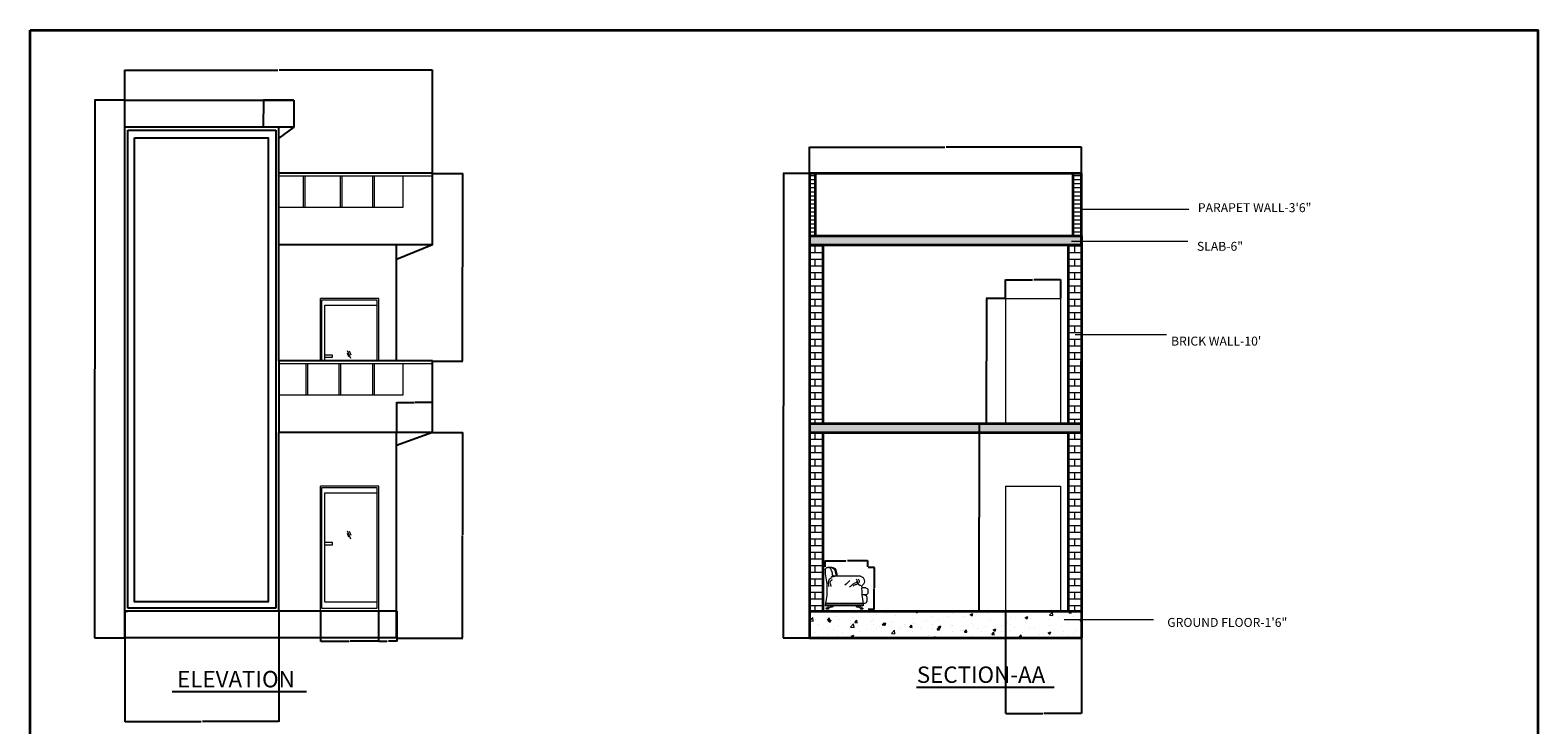
# Model space of a CAD drawing. Units: inches. Extents: x 2169 to 3181, y 1824 to 2912.
# Tile 5 of 5: x 2169 to 3181, y 2446 to 2912. Entities that reach past the tile are written whole.
import ezdxf

# ---------------------------------------------------------------- set-up
doc = ezdxf.new("R2010")
doc.units = ezdxf.units.IN
for name, color, linetype, lineweight in [('A-ANNO-DIMS', 2, 'Continuous', 18), ('A-ANNO-TEXT', 7, 'Continuous', 18), ('A-ANNO-TITL', 7, 'Continuous', 25), ('A-ANNO-TTLB', 7, 'Continuous', 35), ('A-DOOR-ELEV', 3, 'Continuous', 18), ('A-ELEV', 7, 'Continuous', 25), ('A-ELEV-RAIL', 7, 'Continuous', 18), ('A-FLOR-PATT', 252, 'Continuous', 13), ('A-FURN', 8, 'Continuous', 18), ('A-SECT', 7, 'Continuous', 35), ('A-SECT-PRJE', 7, 'Continuous', 18), ('A-WALL-PATT', 252, 'Continuous', 13)]:
    doc.layers.add(name, color=color, linetype=linetype, lineweight=lineweight)
doc.styles.get("Standard").update_dxf_attribs({"font": 'arial.ttf'})
doc.dimstyles.get("Standard").update_dxf_attribs({"dimtxt": 0.18, "dimasz": 0.18, "dimexe": 0.18, "dimexo": 0.0625, "dimgap": 0.09, "dimtad": 0, "dimtih": 1, "dimtoh": 1, "dimdec": 4, "dimzin": 0, "dimdsep": 46, "dimtxsty": 'Standard', "dimcen": 0.09, "dimadec": 0, "dimazin": 0, "dimtfac": 1, "dimtdec": 4, "dimtofl": 0, "dimtmove": 0, "dimatfit": 3, "dimfxl": 1, "dimtolj": 1, "dimtzin": 0, "dimarcsym": 0})

# ---------------------------------------------------------------- blocks, each defined once
blk = doc.blocks.new('A$C624B6646')
for p, q in [((153, 697), (704, 697)), ((161, 698), (700, 698)), ((700, 688), (780, 668)), ((738, 711), (780, 668)), ((769, 889), (830, 881)), ((830, 881), (850, 881)), ((900, 831), (900, 745)), ((0, 400), (0, 350)), ((50, 450), (132, 450)), ((23, 250), (23, 170)), ((50, 300), (125, 300)), ((73, 120), (100, 120)), ((100, 120), (100, 82)), ((100, 82), (900, 82)), ((100, 82), (100, 70)), ((100, 70), (900, 70)), ((104, 120), (900, 120)), ((113, 1), (156, 0)), ((157, 12), (156, 0)), ((166, 27), (157, 12)), ((260, 82), (239, 50)), ((729, 82), (750, 50)), ((823, 27), (832, 12)), ((832, 12), (834, 0)), ((834, 0), (876, 1)), ((900, 82), (900, 70))]:
    blk.add_line(p, q)
for centre, radius, start, end in [((183, 593), 109, 106.2053, 229.88), ((1468, 575), 827, 165.0137, 171.498), ((769, 789), 100, 90, 180), ((1490, 575), 827, 165.0137, 171.498), ((799, 781), 108, 99.7535, 175.837), ((704, 747), 50, 270, 355.0653), ((983, 723), 230, 152.1091, 175.0653), ((830, 831), 50, 90, 180), ((850, 831), 50, 0, 90), ((50, 400), 50, 90, 180), ((50, 350), 50, 180, 270), ((81, 471), 50, 1.791, 49.88), ((73, 250), 50, 90, 180), ((73, 170), 50, 180, 270), ((97, 118), 97.9, 273.831, 296.417), ((118, 16), 15.5, 163.7636, 251.7535), ((230, -4), 95.2, 115.8946, 159.312), ((224, -28), 79.9, 78.8551, 136.1209), ((765, -28), 79.9, 43.8791, 101.1449), ((760, -4), 95.2, 20.688, 64.1054), ((893, 118), 97.9, 243.583, 266.169), ((871, 16), 15.5, 288.2465, 16.2364)]:
    blk.add_arc(centre, radius, start, end)
for points, knots in [([(203, 637), (194, 624), (167, 587), (216, 515), (280, 515), (306, 492), (315, 484)], [0, 0, 0, 0, 46.783568, 128.12179, 194.346234, 229.237423, 229.237423, 229.237423, 229.237423]), ([(245, 644), (235, 621), (212, 571), (298, 543), (345, 504), (373, 475), (385, 463)], [0, 0, 0, 0, 64.284597, 139.770948, 209.553279, 258.887454, 258.887454, 258.887454, 258.887454]), ([(774, 650), (789, 644), (834, 629), (840, 550), (833, 502), (830, 482)], [0, 0, 0, 0, 46.821513, 133.069671, 196.206665, 196.206665, 196.206665, 196.206665]), ([(900, 745), (882, 634), (846, 413), (882, 192), (900, 82)], [0, 0, 0, 0, 336.072717, 666.841786, 666.841786, 666.841786, 666.841786]), ([(147, 498), (162, 501), (194, 507), (223, 553), (219, 586), (217, 602)], [0, 0, 0, 0, 44.149611, 94.447762, 143.253115, 143.253115, 143.253115, 143.253115]), ([(753, 622), (775, 607), (818, 579), (789, 521), (783, 491), (781, 482)], [0, 0, 0, 0, 69.067804, 133.352323, 162.101735, 162.101735, 162.101735, 162.101735])]:
    blk.add_open_spline(points, degree=3, knots=knots)
for points in [[(131, 473), (135, 356), (120, 238), (104, 120)], [(378, 609), (415, 575), (452, 540), (489, 505)]]:
    blk.add_open_spline(points, degree=3)
blk = doc.blocks.new('A$C4C705FAE')
blk.add_blockref('A$C624B6646', (0, 0))
blk = doc.blocks.new('DOOR-OPENING-84IN-SECT')
for p, q in [((0, 84), (37.1, 84)), ((0, 84), (0, 0)), ((37.1, 84), (37.1, 0))]:
    blk.add_line(p, q)
blk = doc.blocks.new('*D49')
at = {"layer": 'A-ANNO-DIMS', "color": 0, "lineweight": -2, "transparency": 16777216}
for p, q in [((2823.3, 2732.3), (2810.6, 2732.3)), ((2810.8, 2732.2), (2810.8, 2690.5)), ((2810.8, 2648.5), (2810.8, 2690.2)), ((2823.3, 2648.3), (2810.6, 2648.3))]:
    blk.add_line(p, q, dxfattribs=at)
at = {"layer": 'A-ANNO-DIMS', "color": 0, "transparency": 16777216}
for points in [[(2810.8, 2732.2), (2810.8, 2732.2), (2810.8, 2732.3)], [(2810.8, 2648.5), (2810.8, 2648.5), (2810.8, 2648.3)]]:
    blk.add_solid(points, dxfattribs=at)
at = {"layer": 'Defpoints', "color": 0, "transparency": 16777216}
for p in [(2810.8, 2732.3), (2823.4, 2732.3), (2823.4, 2648.3)]:
    blk.add_point(p, dxfattribs=at)
at = {"layer": 'A-ANNO-DIMS', "color": 0, "transparency": 16777216, "insert": (2810.8, 2690.3), "char_height": 0.18, "attachment_point": 5}
blk.add_mtext('\\A1;OPENING 84 TYP.', dxfattribs=at)
blk = doc.blocks.new('*D50')
at = {"layer": 'A-ANNO-DIMS', "color": 0, "lineweight": -2, "transparency": 16777216}
for p, q in [((2823.4, 2732.4), (2823.4, 2745.1)), ((2823.6, 2744.9), (2841.5, 2744.9)), ((2860.4, 2744.9), (2842.5, 2744.9)), ((2860.6, 2732.4), (2860.6, 2745.1))]:
    blk.add_line(p, q, dxfattribs=at)
at = {"layer": 'A-ANNO-DIMS', "color": 0, "transparency": 16777216}
for points in [[(2823.6, 2745), (2823.6, 2744.9), (2823.4, 2744.9)], [(2860.4, 2745), (2860.4, 2744.9), (2860.6, 2744.9)]]:
    blk.add_solid(points, dxfattribs=at)
at = {"layer": 'Defpoints', "color": 0, "transparency": 16777216}
for p in [(2860.6, 2744.9), (2823.4, 2732.3), (2860.6, 2732.3)]:
    blk.add_point(p, dxfattribs=at)
at = {"layer": 'A-ANNO-DIMS', "color": 0, "transparency": 16777216, "insert": (2842, 2744.9), "char_height": 0.18, "attachment_point": 5}
blk.add_mtext('\\A1;37 TYP.', dxfattribs=at)
blk = doc.blocks.new('*D51')
at = {"layer": 'A-ANNO-DIMS', "color": 0, "lineweight": -2, "transparency": 16777216}
for p, q in [((2702.5, 2552), (2702.5, 2556.4)), ((2702.7, 2556.2), (2716.2, 2556.2)), ((2730.9, 2556.2), (2717.4, 2556.2)), ((2731.1, 2552), (2731.1, 2556.4))]:
    blk.add_line(p, q, dxfattribs=at)
at = {"layer": 'A-ANNO-DIMS', "color": 0, "transparency": 16777216}
for points in [[(2702.7, 2556.2), (2702.7, 2556.2), (2702.5, 2556.2)], [(2730.9, 2556.2), (2730.9, 2556.2), (2731.1, 2556.2)]]:
    blk.add_solid(points, dxfattribs=at)
at = {"layer": 'Defpoints', "color": 0, "transparency": 16777216}
for p in [(2702.5, 2556.2), (2702.5, 2551.9), (2731.1, 2551.9)]:
    blk.add_point(p, dxfattribs=at)
at = {"layer": 'A-ANNO-DIMS', "color": 0, "transparency": 16777216, "insert": (2716.8, 2556.2), "char_height": 0.18, "attachment_point": 5}
blk.add_mtext('\\A1;CHAIR 29', dxfattribs=at)
blk = doc.blocks.new('*D52')
at = {"layer": 'A-ANNO-DIMS', "color": 0, "lineweight": -2, "transparency": 16777216}
for p, q in [((2731.2, 2551.9), (2735.6, 2551.9)), ((2735.4, 2551.7), (2735.4, 2538)), ((2735.4, 2523.9), (2735.4, 2537.6)), ((2731.2, 2523.7), (2735.6, 2523.7))]:
    blk.add_line(p, q, dxfattribs=at)
at = {"layer": 'A-ANNO-DIMS', "color": 0, "transparency": 16777216}
for points in [[(2735.4, 2551.7), (2735.4, 2551.7), (2735.4, 2551.9)], [(2735.4, 2523.9), (2735.4, 2523.9), (2735.4, 2523.7)]]:
    blk.add_solid(points, dxfattribs=at)
at = {"layer": 'Defpoints', "color": 0, "transparency": 16777216}
for p in [(2731.1, 2551.9), (2735.4, 2551.9), (2731.1, 2523.7)]:
    blk.add_point(p, dxfattribs=at)
at = {"layer": 'A-ANNO-DIMS', "color": 0, "transparency": 16777216, "insert": (2735.4, 2537.8), "char_height": 0.18, "attachment_point": 5}
blk.add_mtext('\\A1;28', dxfattribs=at)
blk = doc.blocks.new('*D71')
at = {"layer": 'A-ANNO-DIMS', "color": 0, "lineweight": -2, "transparency": 16777216}
for p, q in [((2232.2, 2865.5), (2211.9, 2865.5)), ((2212.1, 2865.4), (2212.1, 2685.1)), ((2212.1, 2504.5), (2212.1, 2684.8)), ((2232.2, 2504.3), (2211.9, 2504.3))]:
    blk.add_line(p, q, dxfattribs=at)
at = {"layer": 'A-ANNO-DIMS', "color": 0, "transparency": 16777216}
for points in [[(2212.1, 2865.4), (2212.2, 2865.4), (2212.1, 2865.5)], [(2212.1, 2504.5), (2212.2, 2504.5), (2212.1, 2504.3)]]:
    blk.add_solid(points, dxfattribs=at)
at = {"layer": 'Defpoints', "color": 0, "transparency": 16777216}
for p in [(2212.1, 2865.5), (2232.3, 2865.5), (2232.3, 2504.3)]:
    blk.add_point(p, dxfattribs=at)
at = {"layer": 'A-ANNO-DIMS', "color": 0, "transparency": 16777216, "insert": (2212.1, 2684.9), "char_height": 0.18, "attachment_point": 5}
blk.add_mtext('\\A1;361.2', dxfattribs=at)
blk = doc.blocks.new('*D72')
at = {"layer": 'A-ANNO-DIMS', "color": 0, "lineweight": -2, "transparency": 16777216}
for p, q in [((2232.3, 2865.6), (2232.3, 2885.9)), ((2232.5, 2885.7), (2335.1, 2885.7)), ((2438.6, 2885.7), (2335.9, 2885.7)), ((2438.8, 2816.4), (2438.8, 2885.9))]:
    blk.add_line(p, q, dxfattribs=at)
at = {"layer": 'A-ANNO-DIMS', "color": 0, "transparency": 16777216}
for points in [[(2232.5, 2885.7), (2232.5, 2885.7), (2232.3, 2885.7)], [(2438.6, 2885.7), (2438.6, 2885.7), (2438.8, 2885.7)]]:
    blk.add_solid(points, dxfattribs=at)
at = {"layer": 'Defpoints', "color": 0, "transparency": 16777216}
for p in [(2438.8, 2885.7), (2232.3, 2865.5), (2438.8, 2816.3)]:
    blk.add_point(p, dxfattribs=at)
at = {"layer": 'A-ANNO-DIMS', "color": 0, "transparency": 16777216, "insert": (2335.5, 2885.7), "char_height": 0.18, "attachment_point": 5}
blk.add_mtext('\\A1;206.5', dxfattribs=at)
blk = doc.blocks.new('*D73')
at = {"layer": 'A-ANNO-DIMS', "color": 0, "lineweight": -2, "transparency": 16777216}
for p, q in [((2232.3, 2522.3), (2232.3, 2448)), ((2335.6, 2522.3), (2335.6, 2448)), ((2232.5, 2448.2), (2283.5, 2448.2)), ((2335.5, 2448.2), (2284.4, 2448.2))]:
    blk.add_line(p, q, dxfattribs=at)
at = {"layer": 'A-ANNO-DIMS', "color": 0, "transparency": 16777216}
for points in [[(2232.5, 2448.3), (2232.5, 2448.2), (2232.3, 2448.2)], [(2335.5, 2448.3), (2335.5, 2448.2), (2335.6, 2448.2)]]:
    blk.add_solid(points, dxfattribs=at)
at = {"layer": 'Defpoints', "color": 0, "transparency": 16777216}
for p in [(2232.3, 2522.3), (2335.6, 2522.3), (2335.6, 2448.2)]:
    blk.add_point(p, dxfattribs=at)
at = {"layer": 'A-ANNO-DIMS', "color": 0, "transparency": 16777216, "insert": (2284, 2448.2), "char_height": 0.18, "attachment_point": 5}
blk.add_mtext('\\A1;103.36', dxfattribs=at)
blk = doc.blocks.new('*D74')
at = {"layer": 'A-ANNO-DIMS', "color": 0, "lineweight": -2, "transparency": 16777216}
for p, q in [((2438.8, 2816.3), (2459.1, 2816.3)), ((2458.9, 2816.2), (2458.9, 2753.5)), ((2458.9, 2690.5), (2458.9, 2753.2)), ((2438.8, 2690.3), (2459.1, 2690.3))]:
    blk.add_line(p, q, dxfattribs=at)
at = {"layer": 'A-ANNO-DIMS', "color": 0, "transparency": 16777216}
for points in [[(2458.9, 2816.2), (2459, 2816.2), (2458.9, 2816.3)], [(2458.9, 2690.5), (2459, 2690.5), (2458.9, 2690.3)]]:
    blk.add_solid(points, dxfattribs=at)
at = {"layer": 'Defpoints', "color": 0, "transparency": 16777216}
for p in [(2438.8, 2816.3), (2458.9, 2816.3), (2438.8, 2690.3)]:
    blk.add_point(p, dxfattribs=at)
at = {"layer": 'A-ANNO-DIMS', "color": 0, "transparency": 16777216, "insert": (2458.9, 2753.3), "char_height": 0.18, "attachment_point": 5}
blk.add_mtext('\\A1;126', dxfattribs=at)
blk = doc.blocks.new('*D75')
at = {"layer": 'A-ANNO-DIMS', "color": 0, "lineweight": -2, "transparency": 16777216}
for p, q in [((2438.8, 2642.3), (2459.1, 2642.3)), ((2458.9, 2642.2), (2458.9, 2573.5)), ((2458.9, 2504.5), (2458.9, 2573.2)), ((2414.8, 2504.3), (2459.1, 2504.3))]:
    blk.add_line(p, q, dxfattribs=at)
at = {"layer": 'A-ANNO-DIMS', "color": 0, "transparency": 16777216}
for points in [[(2458.9, 2642.2), (2459, 2642.2), (2458.9, 2642.3)], [(2458.9, 2504.5), (2459, 2504.5), (2458.9, 2504.3)]]:
    blk.add_solid(points, dxfattribs=at)
at = {"layer": 'Defpoints', "color": 0, "transparency": 16777216}
for p in [(2438.8, 2642.3), (2458.9, 2642.3), (2414.8, 2504.3)]:
    blk.add_point(p, dxfattribs=at)
at = {"layer": 'A-ANNO-DIMS', "color": 0, "transparency": 16777216, "insert": (2458.9, 2573.3), "char_height": 0.18, "attachment_point": 5}
blk.add_mtext('\\A1;138', dxfattribs=at)
blk = doc.blocks.new('*D76')
at = {"layer": 'A-ANNO-DIMS', "color": 0, "lineweight": -2, "transparency": 16777216}
for p, q in [((2414.8, 2642.4), (2414.8, 2662.7)), ((2415, 2662.5), (2426.6, 2662.5)), ((2438.6, 2662.5), (2427, 2662.5)), ((2438.8, 2642.4), (2438.8, 2662.7))]:
    blk.add_line(p, q, dxfattribs=at)
at = {"layer": 'A-ANNO-DIMS', "color": 0, "transparency": 16777216}
for points in [[(2415, 2662.5), (2415, 2662.5), (2414.8, 2662.5)], [(2438.6, 2662.5), (2438.6, 2662.5), (2438.8, 2662.5)]]:
    blk.add_solid(points, dxfattribs=at)
at = {"layer": 'Defpoints', "color": 0, "transparency": 16777216}
for p in [(2438.8, 2662.5), (2414.8, 2642.3), (2438.8, 2642.3)]:
    blk.add_point(p, dxfattribs=at)
at = {"layer": 'A-ANNO-DIMS', "color": 0, "transparency": 16777216, "insert": (2426.8, 2662.5), "char_height": 0.18, "attachment_point": 5}
blk.add_mtext('\\A1;24', dxfattribs=at)
blk = doc.blocks.new('*D77')
at = {"layer": 'A-ANNO-DIMS', "color": 0, "lineweight": -2, "transparency": 16777216}
for p, q in [((2402.7, 2522.3), (2402.7, 2502)), ((2414.8, 2522.3), (2414.8, 2502)), ((2402.9, 2502.2), (2408.3, 2502.2)), ((2414.6, 2502.2), (2409.2, 2502.2))]:
    blk.add_line(p, q, dxfattribs=at)
at = {"layer": 'A-ANNO-DIMS', "color": 0, "transparency": 16777216}
for points in [[(2402.9, 2502.2), (2402.9, 2502.2), (2402.7, 2502.2)], [(2414.6, 2502.2), (2414.6, 2502.2), (2414.8, 2502.2)]]:
    blk.add_solid(points, dxfattribs=at)
at = {"layer": 'Defpoints', "color": 0, "transparency": 16777216}
for p in [(2402.7, 2522.3), (2414.8, 2522.3), (2402.7, 2502.2)]:
    blk.add_point(p, dxfattribs=at)
at = {"layer": 'A-ANNO-DIMS', "color": 0, "transparency": 16777216, "insert": (2408.8, 2502.2), "char_height": 0.18, "attachment_point": 5}
blk.add_mtext('\\A1;12.041', dxfattribs=at)
blk = doc.blocks.new('*D78')
at = {"layer": 'A-ANNO-DIMS', "color": 0, "lineweight": -2, "transparency": 16777216}
for p, q in [((2363.7, 2522.3), (2363.7, 2502)), ((2402.7, 2522.3), (2402.7, 2502)), ((2363.9, 2502.2), (2382.9, 2502.2)), ((2402.6, 2502.2), (2383.6, 2502.2))]:
    blk.add_line(p, q, dxfattribs=at)
at = {"layer": 'A-ANNO-DIMS', "color": 0, "transparency": 16777216}
for points in [[(2363.9, 2502.2), (2363.9, 2502.2), (2363.7, 2502.2)], [(2402.6, 2502.2), (2402.6, 2502.2), (2402.7, 2502.2)]]:
    blk.add_solid(points, dxfattribs=at)
at = {"layer": 'Defpoints', "color": 0, "transparency": 16777216}
for p in [(2363.7, 2522.3), (2402.7, 2522.3), (2363.7, 2502.2)]:
    blk.add_point(p, dxfattribs=at)
at = {"layer": 'A-ANNO-DIMS', "color": 0, "transparency": 16777216, "insert": (2383.2, 2502.2), "char_height": 0.18, "attachment_point": 5}
blk.add_mtext('\\A1;39.01', dxfattribs=at)
blk = doc.blocks.new('*D79')
at = {"layer": 'A-ANNO-DIMS', "color": 0, "lineweight": -2, "transparency": 16777216}
for p, q in [((2345.6, 2865.5), (2325.4, 2865.5)), ((2325.5, 2865.4), (2325.5, 2856.6)), ((2325.5, 2847.5), (2325.5, 2856.3)), ((2345.6, 2847.3), (2325.4, 2847.3))]:
    blk.add_line(p, q, dxfattribs=at)
at = {"layer": 'A-ANNO-DIMS', "color": 0, "transparency": 16777216}
for points in [[(2325.5, 2865.4), (2325.6, 2865.4), (2325.5, 2865.5)], [(2325.5, 2847.5), (2325.6, 2847.5), (2325.5, 2847.3)]]:
    blk.add_solid(points, dxfattribs=at)
at = {"layer": 'Defpoints', "color": 0, "transparency": 16777216}
for p in [(2325.5, 2865.5), (2345.7, 2865.5), (2345.7, 2847.3)]:
    blk.add_point(p, dxfattribs=at)
at = {"layer": 'A-ANNO-DIMS', "color": 0, "transparency": 16777216, "insert": (2325.5, 2856.4), "char_height": 0.18, "attachment_point": 5}
blk.add_mtext('\\A1;18.2', dxfattribs=at)
blk = doc.blocks.new('*D80')
at = {"layer": 'A-ANNO-DIMS', "color": 0, "lineweight": -2, "transparency": 16777216}
for p, q in [((2692, 2816.4), (2692, 2834.1)), ((2692.1, 2833.9), (2782.8, 2833.9)), ((2874.3, 2833.9), (2783.6, 2833.9)), ((2874.5, 2816.4), (2874.5, 2834.1))]:
    blk.add_line(p, q, dxfattribs=at)
at = {"layer": 'A-ANNO-DIMS', "color": 0, "transparency": 16777216}
for points in [[(2692.1, 2833.9), (2692.1, 2833.9), (2692, 2833.9)], [(2874.3, 2833.9), (2874.3, 2833.9), (2874.5, 2833.9)]]:
    blk.add_solid(points, dxfattribs=at)
at = {"layer": 'Defpoints', "color": 0, "transparency": 16777216}
for p in [(2874.5, 2833.9), (2692, 2816.3), (2874.5, 2816.3)]:
    blk.add_point(p, dxfattribs=at)
at = {"layer": 'A-ANNO-DIMS', "color": 0, "transparency": 16777216, "insert": (2783.2, 2833.9), "char_height": 0.18, "attachment_point": 5}
blk.add_mtext('\\A1;182.5', dxfattribs=at)
blk = doc.blocks.new('*D81')
at = {"layer": 'A-ANNO-DIMS', "color": 0, "lineweight": -2, "transparency": 16777216}
for p, q in [((2691.9, 2816.3), (2674.2, 2816.3)), ((2674.4, 2816.2), (2674.4, 2660.5)), ((2674.4, 2504.5), (2674.4, 2660.2)), ((2691.9, 2504.3), (2674.2, 2504.3))]:
    blk.add_line(p, q, dxfattribs=at)
at = {"layer": 'A-ANNO-DIMS', "color": 0, "transparency": 16777216}
for points in [[(2674.4, 2816.2), (2674.4, 2816.2), (2674.4, 2816.3)], [(2674.4, 2504.5), (2674.4, 2504.5), (2674.4, 2504.3)]]:
    blk.add_solid(points, dxfattribs=at)
at = {"layer": 'Defpoints', "color": 0, "transparency": 16777216}
for p in [(2674.4, 2816.3), (2692, 2816.3), (2692, 2504.3)]:
    blk.add_point(p, dxfattribs=at)
at = {"layer": 'A-ANNO-DIMS', "color": 0, "transparency": 16777216, "insert": (2674.4, 2660.3), "char_height": 0.18, "attachment_point": 5}
blk.add_mtext('\\A1;312', dxfattribs=at)
blk = doc.blocks.new('*D82')
at = {"layer": 'A-ANNO-DIMS', "color": 0, "lineweight": -2, "transparency": 16777216}
for p, q in [((2823.3, 2648.3), (2805.7, 2648.3)), ((2805.9, 2648.2), (2805.9, 2585.5)), ((2805.9, 2522.5), (2805.9, 2585.2)), ((2823.3, 2522.3), (2805.7, 2522.3))]:
    blk.add_line(p, q, dxfattribs=at)
at = {"layer": 'A-ANNO-DIMS', "color": 0, "transparency": 16777216}
for points in [[(2805.8, 2648.2), (2805.9, 2648.2), (2805.9, 2648.3)], [(2805.8, 2522.5), (2805.9, 2522.5), (2805.9, 2522.3)]]:
    blk.add_solid(points, dxfattribs=at)
at = {"layer": 'Defpoints', "color": 0, "transparency": 16777216}
for p in [(2805.9, 2648.3), (2823.4, 2648.3), (2823.4, 2522.3)]:
    blk.add_point(p, dxfattribs=at)
at = {"layer": 'A-ANNO-DIMS', "color": 0, "transparency": 16777216, "insert": (2805.9, 2585.3), "char_height": 0.18, "attachment_point": 5}
blk.add_mtext('\\A1;126', dxfattribs=at)
blk = doc.blocks.new('*D83')
at = {"layer": 'A-ANNO-DIMS', "color": 0, "lineweight": -2, "transparency": 16777216}
for p, q in [((2823.4, 2522.3), (2823.4, 2453.5)), ((2874.5, 2504.3), (2874.5, 2453.5)), ((2823.6, 2453.7), (2848.5, 2453.7)), ((2874.3, 2453.7), (2849.3, 2453.7))]:
    blk.add_line(p, q, dxfattribs=at)
at = {"layer": 'A-ANNO-DIMS', "color": 0, "transparency": 16777216}
for points in [[(2823.6, 2453.7), (2823.6, 2453.7), (2823.4, 2453.7)], [(2874.3, 2453.7), (2874.3, 2453.7), (2874.5, 2453.7)]]:
    blk.add_solid(points, dxfattribs=at)
at = {"layer": 'Defpoints', "color": 0, "transparency": 16777216}
for p in [(2823.4, 2522.3), (2874.5, 2504.3), (2823.4, 2453.7)]:
    blk.add_point(p, dxfattribs=at)
at = {"layer": 'A-ANNO-DIMS', "color": 0, "transparency": 16777216, "insert": (2848.9, 2453.7), "char_height": 0.18, "attachment_point": 5}
blk.add_mtext('\\A1;51.05', dxfattribs=at)

msp = doc.modelspace()

# ---------------------------------------------------------------- hatches: boundary and pattern name
at = {"layer": 'A-FLOR-PATT'}
h = msp.add_hatch(dxfattribs=at)
h.set_pattern_fill('AR-CONC', color=256, scale=0.042, style=0)
h.paths.add_polyline_path([(2691.9572, 2768.3402), (2874.4572, 2768.3402), (2874.4572, 2774.3402), (2691.9572, 2774.3402)])
h = msp.add_hatch(dxfattribs=at)
h.set_pattern_fill('AR-CONC', color=256, scale=0.042, style=0)
h.paths.add_polyline_path([(2691.9572, 2642.3402), (2874.4572, 2642.3402), (2874.4572, 2648.3402), (2691.9572, 2648.3402)])
h = msp.add_hatch(dxfattribs=at)
h.set_pattern_fill('AR-CONC', color=256, scale=0.101, style=0)
h.paths.add_polyline_path([(2691.9572, 2504.3402), (2874.4572, 2504.3402), (2874.4572, 2522.3402), (2691.9572, 2522.3402)])
at = {"layer": 'A-WALL-PATT'}
h = msp.add_hatch(dxfattribs=at)
h.set_pattern_fill('LINE', color=256, scale=0.85, style=0)
h.paths.add_polyline_path([(2691.9572, 2774.3402), (2695.9125, 2774.3402), (2695.9125, 2816.3402), (2691.9572, 2816.3402)])
h = msp.add_hatch(dxfattribs=at)
h.set_pattern_fill('LINE', color=256, scale=0.85, style=0)
h.paths.add_polyline_path([(2868.9519, 2774.3402), (2874.4572, 2774.3402), (2874.4572, 2816.3402), (2868.9519, 2816.3402)])
h = msp.add_hatch(dxfattribs=at)
h.set_pattern_fill('AR-BRSTD', color=256, scale=0.066, style=0)
h.paths.add_polyline_path([(2691.9572, 2648.3402), (2700.9572, 2648.3402), (2700.9572, 2768.3402), (2691.9572, 2768.3402)])
h = msp.add_hatch(dxfattribs=at)
h.set_pattern_fill('AR-BRSTD', color=256, scale=0.066, style=0)
h.paths.add_polyline_path([(2865.4572, 2648.3402), (2874.4572, 2648.3402), (2874.4572, 2768.3402), (2865.4572, 2768.3402)])
h = msp.add_hatch(dxfattribs=at)
h.set_pattern_fill('AR-BRSTD', color=256, scale=0.066, style=0)
h.paths.add_polyline_path([(2691.9572, 2522.3402), (2700.9572, 2522.3402), (2700.9572, 2642.3402), (2691.9572, 2642.3402)])
h = msp.add_hatch(dxfattribs=at)
h.set_pattern_fill('AR-BRSTD', color=256, scale=0.066, style=0)
h.paths.add_polyline_path([(2865.4572, 2522.3402), (2874.4572, 2522.3402), (2874.4572, 2642.3402), (2865.4572, 2642.3402)])

# ---------------------------------------------------------------- linework, layer by layer
at = {"layer": 'A-ANNO-TEXT'}
for p, q in [((2874.4572, 2792.3402), (2946.4972, 2792.3402)), ((2867.7172, 2770.7123), (2945.9368, 2770.7123)), ((2870.1556, 2708.1716), (2931.5391, 2708.1716)), ((2862.8948, 2516.6543), (2922.8793, 2516.6543))]:
    msp.add_line(p, q, dxfattribs=at)
at = {"layer": 'A-ANNO-TITL'}
for p, q in [((2763.6385, 2471.2423), (2856.1799, 2471.2423)), ((2264.0822, 2468.3701), (2354.3391, 2468.3701)), ((2354.3391, 2468.3701), (2354.3391, 2468.3701))]:
    msp.add_line(p, q, dxfattribs=at)
at = {"layer": 'A-ANNO-TTLB'}
msp.add_lwpolyline([(2168.7598, 2912.462), (3180.8253, 2912.462), (3180.8253, 1823.5481), (2168.7598, 1823.5481)], close=True, dxfattribs=at)
at = {"layer": 'A-DOOR-ELEV'}
for p, q in [((2363.7249, 2690.3402), (2363.7249, 2732.3402)), ((2402.7324, 2732.3402), (2363.7249, 2732.3402)), ((2363.7249, 2690.3402), (2363.7249, 2732.3402)), ((2402.7324, 2732.3402), (2363.7249, 2732.3402)), ((2402.7324, 2690.3402), (2402.7324, 2732.3402)), ((2402.7324, 2690.3402), (2402.7324, 2732.3402)), ((2381.5185, 2695.8064), (2382.3485, 2693.3994)), ((2381.6432, 2697.4153), (2383.7338, 2692.1256)), ((2382.968, 2697.2203), (2383.985, 2694.4978)), ((2402.7324, 2606.3402), (2363.7249, 2606.3402)), ((2363.7249, 2522.3402), (2363.7249, 2606.3402)), ((2402.7324, 2522.3402), (2402.7324, 2606.3402)), ((2381.5185, 2574.6444), (2382.3485, 2572.2374)), ((2381.6432, 2576.2532), (2383.7338, 2570.9636)), ((2382.968, 2576.0582), (2383.985, 2573.3357))]:
    msp.add_line(p, q, dxfattribs=at)
for points in [[(2364.5198, 2690.3402), (2364.5198, 2731.4024), (2401.4324, 2731.4024), (2401.4324, 2690.3402)], [(2366.5527, 2690.3402), (2366.5527, 2727.7588), (2401.4324, 2727.7588), (2401.4324, 2690.3402)]]:
    msp.add_lwpolyline(points, dxfattribs=at)
for points in [[(2366.5527, 2694.5414), (2371.5246, 2694.5414), (2371.5246, 2692.6612), (2366.5527, 2692.6612)], [(2364.5198, 2605.4024), (2401.4324, 2605.4024), (2401.4324, 2524.0403), (2364.5198, 2524.0403)], [(2366.5527, 2601.7588), (2401.4324, 2601.7588), (2401.4324, 2528.4361), (2366.5527, 2528.4361)], [(2366.5527, 2568.5414), (2371.5246, 2568.5414), (2371.5246, 2566.6612), (2366.5527, 2566.6612)]]:
    msp.add_lwpolyline(points, close=True, dxfattribs=at)
at = {"layer": 'A-ELEV'}
for p, q in [((2232.2736, 2642.3402), (2232.2736, 2865.5383)), ((2232.2736, 2865.5383), (2335.637, 2865.5383)), ((2335.637, 2865.5383), (2345.6981, 2865.5383)), ((2345.6981, 2865.5383), (2345.6981, 2847.3388)), ((2335.637, 2847.3388), (2232.2736, 2847.3388)), ((2234.2736, 2524.3402), (2234.2736, 2845.3388)), ((2234.2736, 2845.3388), (2333.637, 2845.3388)), ((2333.637, 2845.3388), (2333.637, 2524.3402)), ((2335.637, 2768.3402), (2335.637, 2847.3388)), ((2345.6981, 2847.3388), (2335.637, 2847.3388)), ((2345.6981, 2847.3388), (2335.637, 2839.8437)), ((2438.7736, 2816.3402), (2335.637, 2816.3402)), ((2438.7736, 2768.3402), (2438.7736, 2816.3402)), ((2232.2736, 2690.3402), (2232.2736, 2768.3402)), ((2232.2736, 2690.3402), (2232.2736, 2768.3402)), ((2335.637, 2690.3402), (2335.637, 2768.3402)), ((2438.7736, 2768.3402), (2335.637, 2768.3402)), ((2414.7736, 2690.3402), (2414.7736, 2768.3402)), ((2438.7736, 2768.3402), (2414.7736, 2758.3597)), ((2438.7736, 2690.3402), (2335.637, 2690.3402)), ((2335.637, 2690.3402), (2335.637, 2690.3402)), ((2335.637, 2690.3402), (2335.637, 2642.3402)), ((2438.7736, 2642.3402), (2438.7736, 2690.3402)), ((2232.2736, 2504.3402), (2232.2736, 2642.3402)), ((2232.2736, 2504.3402), (2232.2736, 2642.3402)), ((2232.2736, 2630.3402), (2232.2736, 2642.3402)), ((2232.2736, 2630.3402), (2232.2736, 2642.3402)), ((2232.2736, 2642.3402), (2232.2736, 2642.3402)), ((2438.7736, 2642.3402), (2335.637, 2642.3402)), ((2335.637, 2522.3402), (2335.637, 2642.3402)), ((2414.7736, 2504.3402), (2414.7736, 2642.3402)), ((2414.7736, 2630.3402), (2414.7736, 2642.3402)), ((2438.7736, 2642.3402), (2414.7736, 2633.5534)), ((2414.7736, 2633.5534), (2414.7736, 2633.5534)), ((2414.7736, 2522.3402), (2232.2736, 2522.3402)), ((2232.2736, 2522.3402), (2234.2736, 2522.3402)), ((2333.637, 2524.3402), (2234.2736, 2524.3402)), ((2414.7736, 2504.3402), (2232.2736, 2504.3402))]:
    msp.add_line(p, q, dxfattribs=at)
msp.add_lwpolyline([(2238.7786, 2840.2302), (2328.5033, 2840.2302), (2328.5033, 2528.5906), (2238.7786, 2528.5906)], close=True, dxfattribs=at)
at = {"layer": 'A-ELEV-RAIL'}
for p, q in [((2438.7736, 2814.3402), (2335.637, 2814.3402)), ((2352.1576, 2793.2915), (2352.1576, 2814.3402)), ((2353.1576, 2814.3402), (2353.1576, 2793.2915)), ((2377.0694, 2793.2915), (2377.0694, 2814.3402)), ((2378.0694, 2814.3402), (2378.0694, 2793.2915)), ((2398.7296, 2793.2915), (2398.7296, 2814.3402)), ((2399.7296, 2814.3402), (2399.7296, 2793.2915)), ((2418.9004, 2814.3402), (2418.9004, 2793.2915)), ((2438.7736, 2816.3402), (2438.7736, 2814.3402)), ((2418.9004, 2793.2915), (2335.637, 2793.2915)), ((2399.7296, 2793.2915), (2398.7296, 2793.2915)), ((2438.7736, 2690.3402), (2335.637, 2690.3402)), ((2438.7736, 2688.3402), (2335.637, 2688.3402)), ((2438.7736, 2688.3402), (2335.637, 2688.3402)), ((2354.0166, 2667.2915), (2354.0166, 2688.3402)), ((2355.0166, 2688.3402), (2355.0166, 2667.2915)), ((2376.1749, 2667.2915), (2376.1749, 2688.3402)), ((2377.1749, 2688.3402), (2377.1749, 2667.2915)), ((2398.7296, 2667.2915), (2398.7296, 2688.3402)), ((2399.7296, 2688.3402), (2399.7296, 2667.2915)), ((2418.9004, 2688.3402), (2418.9004, 2667.2915)), ((2438.7736, 2690.3402), (2438.7736, 2688.3402)), ((2418.9004, 2667.2915), (2335.637, 2667.2915)), ((2399.7296, 2667.2915), (2398.7296, 2667.2915))]:
    msp.add_line(p, q, dxfattribs=at)
at = {"layer": 'A-SECT'}
for p, q in [((2691.9572, 2816.3402), (2691.9572, 2630.3402)), ((2691.9572, 2816.3402), (2874.4572, 2816.3402)), ((2695.9125, 2774.3402), (2695.9125, 2816.3402)), ((2868.9519, 2774.3402), (2868.9519, 2816.3402)), ((2874.4572, 2768.3402), (2874.4572, 2816.3402)), ((2691.9572, 2774.3402), (2874.4572, 2774.3402)), ((2874.4572, 2774.3402), (2874.4572, 2630.3402)), ((2691.9572, 2768.3402), (2874.4572, 2768.3402)), ((2700.9572, 2768.3402), (2700.9572, 2648.3402)), ((2865.4572, 2768.3402), (2865.4572, 2648.3402)), ((2691.9572, 2690.3402), (2691.9572, 2504.3402)), ((2874.4572, 2642.3402), (2874.4572, 2690.3402)), ((2691.9572, 2648.3402), (2874.4572, 2648.3402)), ((2691.9572, 2642.3402), (2874.4572, 2642.3402)), ((2700.9572, 2642.3402), (2700.9572, 2522.3402)), ((2865.4572, 2642.3402), (2865.4572, 2522.3402)), ((2874.4572, 2648.3402), (2874.4572, 2504.3402)), ((2691.9572, 2522.3402), (2874.4572, 2522.3402)), ((2691.9572, 2504.3402), (2874.4572, 2504.3402))]:
    msp.add_line(p, q, dxfattribs=at)

# ---------------------------------------------------------------- block references
at = {"layer": 'A-FURN', "xscale": -0.0317727134028724, "yscale": 0.0317727134028724, "zscale": 0.0317727134028724}
msp.add_blockref('A$C4C705FAE', (2731.1024, 2523.6713), dxfattribs=at)
at = {"layer": 'A-SECT-PRJE'}
for p in [(2823.408, 2648.34), (2823.408, 2522.34)]:
    msp.add_blockref('DOOR-OPENING-84IN-SECT', p, dxfattribs=at)

# ---------------------------------------------------------------- texts
at = {"layer": 'A-ANNO-TEXT', "char_height": 6, "attachment_point": 1}
for s, width, insert in [('PARAPET WALL-3\'6"', 161.914669, (2952.5997, 2796.2732)), ('SLAB-6"', 70.888526, (2951.9923, 2770.3103)), ("BRICK WALL-10'", 94.222954, (2934.613, 2706.6676)), ('GROUND FLOOR-1\'6"', 137.072599, (2932.0565, 2517.7701))]:
    msp.add_mtext_dynamic_manual_height_columns(s, width=width, gutter_width=12.5, heights=[0], dxfattribs=dict(at, insert=insert))
at = {"layer": 'A-ANNO-TITL', "char_height": 11, "attachment_point": 1}
for s, width, insert in [('ELEVATION', 238.845284, (2267.4481, 2482.1703)), ('SECTION-AA', 405.672923, (2763.9539, 2485.1722))]:
    msp.add_mtext_dynamic_manual_height_columns(s, width=width, gutter_width=12.5, heights=[0], dxfattribs=dict(at, insert=insert))

# ---------------------------------------------------------------- dimensions: what is measured, and where the dimension line sits
at = {"layer": 'A-ANNO-DIMS'}
for base, p1, p2, override, picture, middle in [((2438.7736, 2885.6883), (2232.2736, 2865.5383), (2438.7736, 2816.3402), {"dimdec": 1, "dimlfac": 1, "dimrnd": 0, "dimzin": 0, "dimdsep": 46, "dimlunit": 2}, '*D72', (2335.5236, 2885.6883)), ((2874.4572, 2833.8902), (2691.9572, 2816.3402), (2874.4572, 2816.3402), {"dimdec": 1, "dimlfac": 1, "dimrnd": 0, "dimzin": 0, "dimdsep": 46, "dimlunit": 2}, '*D80', (2783.2072, 2833.8902)), ((2335.637, 2448.2201), (2232.2736, 2522.3402), (2335.637, 2522.3402), {"dimdec": 2, "dimlfac": 1, "dimrnd": 0, "dimzin": 0, "dimdsep": 46, "dimlunit": 2}, '*D73', (2283.9553, 2448.2201)), ((2823.4085, 2453.6923), (2874.4572, 2504.3402), (2823.4085, 2522.3402), {"dimdec": 2, "dimlfac": 1, "dimrnd": 0, "dimzin": 0, "dimdsep": 46, "dimlunit": 2}, '*D83', (2848.9329, 2453.6923))]:
    dim = msp.add_linear_dim(base=base, p1=p1, p2=p2, dimstyle='Standard', override=override, dxfattribs=at)
    dim.commit()
    dim.dimension.update_dxf_attribs({"geometry": picture, "text_midpoint": middle})
for base, p1, p2, angle, override, picture, middle in [((2212.1236, 2865.5383), (2232.2736, 2504.3402), (2232.2736, 2865.5383), 90, {"dimdec": 1, "dimlfac": 1, "dimrnd": 0, "dimzin": 0, "dimdsep": 46, "dimlunit": 2}, '*D71', (2212.1236, 2684.9392)), ((2325.5481, 2865.5383), (2345.6981, 2847.3388), (2345.6981, 2865.5383), 90, {"dimdec": 1, "dimlfac": 1, "dimrnd": 0, "dimzin": 0, "dimdsep": 46, "dimlunit": 2}, '*D79', (2325.5481, 2856.4386)), ((2458.9236, 2816.3402), (2438.7736, 2690.3402), (2438.7736, 2816.3402), 90, {"dimdec": 0, "dimlfac": 1, "dimrnd": 0, "dimzin": 0, "dimdsep": 46, "dimlunit": 2}, '*D74', (2458.9236, 2753.3402)), ((2674.4072, 2816.3402), (2691.9572, 2504.3402), (2691.9572, 2816.3402), 90, {"dimdec": 0, "dimlfac": 1, "dimrnd": 0, "dimzin": 0, "dimdsep": 46, "dimlunit": 2}, '*D81', (2674.4072, 2660.3402)), ((2438.7736, 2662.4902), (2414.7736, 2642.3402), (2438.7736, 2642.3402), 0, {"dimdec": 0, "dimlfac": 1, "dimrnd": 0, "dimzin": 0, "dimdsep": 46, "dimlunit": 2}, '*D76', (2426.7736, 2662.4902)), ((2458.9236, 2642.3402), (2414.7736, 2504.3402), (2438.7736, 2642.3402), 90, {"dimdec": 0, "dimlfac": 1, "dimrnd": 0, "dimzin": 0, "dimdsep": 46, "dimlunit": 2}, '*D75', (2458.9236, 2573.3402)), ((2805.8585, 2648.3402), (2823.4085, 2522.3402), (2823.4085, 2648.3402), 90, {"dimdec": 0, "dimlfac": 1, "dimrnd": 0, "dimzin": 0, "dimdsep": 46, "dimlunit": 2}, '*D82', (2805.8585, 2585.3402)), ((2735.3917, 2551.915), (2731.1024, 2523.6713), (2731.1024, 2551.915), 90, {"dimdec": 0, "dimlfac": 1, "dimrnd": 0, "dimzin": 0, "dimdsep": 46, "dimlunit": 2}, '*D52', (2735.3917, 2537.7931)), ((2363.7249, 2502.1902), (2402.7324, 2522.3402), (2363.7249, 2522.3402), 180, {"dimdec": 2, "dimlfac": 1, "dimrnd": 0, "dimzin": 0, "dimdsep": 46, "dimlunit": 2}, '*D78', (2383.2286, 2502.1902)), ((2402.7324, 2502.1902), (2414.7736, 2522.3402), (2402.7324, 2522.3402), 180, {"dimdec": 3, "dimlfac": 1, "dimrnd": 0, "dimzin": 0, "dimdsep": 46, "dimlunit": 2}, '*D77', (2408.753, 2502.1902))]:
    dim = msp.add_linear_dim(base=base, p1=p1, p2=p2, angle=angle, dimstyle='Standard', override=override, dxfattribs=at)
    dim.commit()
    dim.dimension.update_dxf_attribs({"geometry": picture, "text_midpoint": middle})
dim = msp.add_linear_dim(base=(2860.5569, 2744.9402), p1=(2823.4085, 2732.3402), p2=(2860.5569, 2732.3402), text='<> TYP.', dimstyle='Standard', override={"dimdec": 0, "dimlfac": 1, "dimrnd": 0, "dimzin": 0, "dimdsep": 46, "dimlunit": 2}, dxfattribs=at)
dim.commit()
dim.dimension.update_dxf_attribs({"geometry": '*D50', "text_midpoint": (2841.9827, 2744.9402)})
for base, p1, p2, angle, text, picture, middle in [((2810.8085, 2732.3402), (2823.4085, 2648.3402), (2823.4085, 2732.3402), 90, 'OPENING <> TYP.', '*D49', (2810.8085, 2690.3402)), ((2702.5069, 2556.2043), (2731.1024, 2551.915), (2702.5069, 2551.915), 180, 'CHAIR <>', '*D51', (2716.8046, 2556.2043))]:
    dim = msp.add_linear_dim(base=base, p1=p1, p2=p2, angle=angle, text=text, dimstyle='Standard', override={"dimdec": 0, "dimlfac": 1, "dimrnd": 0, "dimzin": 0, "dimdsep": 46, "dimlunit": 2}, dxfattribs=at)
    dim.commit()
    dim.dimension.update_dxf_attribs({"geometry": picture, "text_midpoint": middle})

doc.saveas('drawing.dxf')
